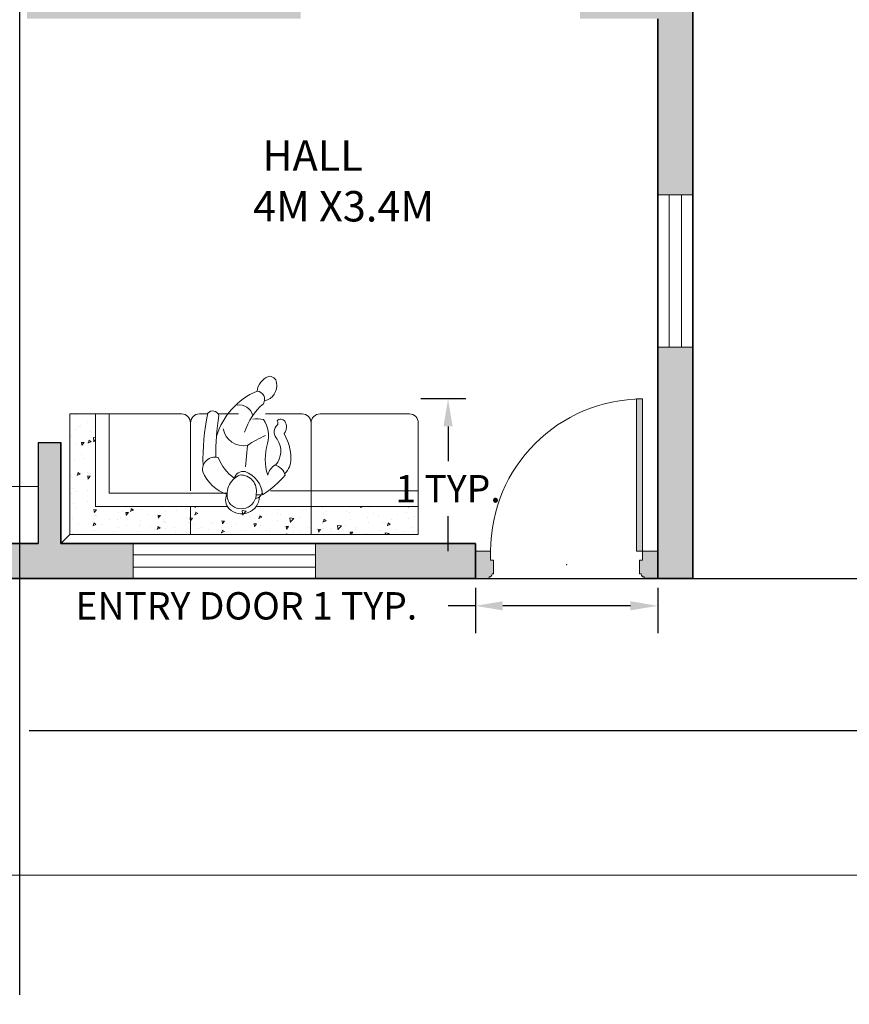
# Model space of a CAD drawing. Units: metres. Extents: x 2031 to 2061.8, y 1886.4 to 1909.8.
# Tile 5 of 10: x 2040.4 to 2045.9, y 1896.6 to 1903. Entities that reach past the tile are written whole.
import ezdxf

# ---------------------------------------------------------------- set-up
doc = ezdxf.new("R2010")
doc.units = ezdxf.units.M
for name, color, linetype, lineweight in [('A-ANNO-DIMS', 2, 'Continuous', 18), ('A-ANNO-SYMB', 7, 'Continuous', 18), ('A-AREA-IDEN', 7, 'Continuous', 18), ('A-FLOR-CASE', 8, 'Continuous', 18), ('A-WALL-PATT', 252, 'Continuous', 13), ('doors & windows', 30, 'Continuous', 18), ('furniture', 24, 'Continuous', 13), ('inner walls', 4, 'Continuous', 25), ('windows', 30, 'Continuous', 18)]:
    doc.layers.add(name, color=color, linetype=linetype, lineweight=lineweight)
doc.layers.add('outer walls', color=1, linetype='Continuous', lineweight=35, plot=False)
doc.styles.get("Standard").update_dxf_attribs({"font": 'arial.ttf'})
doc.dimstyles.get("Standard").update_dxf_attribs({"dimtxt": 0.18, "dimasz": 0.18, "dimexe": 0.18, "dimexo": 0.0625, "dimgap": 0.09, "dimtad": 0, "dimtih": 1, "dimtoh": 1, "dimdec": 4, "dimzin": 0, "dimdsep": 46, "dimtxsty": 'Standard', "dimcen": 0.09, "dimadec": 0, "dimazin": 0, "dimtfac": 1, "dimtdec": 4, "dimtofl": 0, "dimtmove": 0, "dimatfit": 3, "dimfxl": 1, "dimtolj": 1, "dimtzin": 0, "dimarcsym": 0})

# ---------------------------------------------------------------- blocks, each defined once
blk = doc.blocks.new('MAN')
at = {"layer": 'doors & windows'}
blk.add_line((1.300800906350296, -9.84959528513384), (0.8904374767287208, -5.445845033773593), dxfattribs=at)
for centre, radius, start, end in [((0.1037123764109868, 0.4753156361215943), 3.598756859045963, 2.892834703444422, 134.5528130484283), ((-0.8140254724787943, 1.304327540725086), 2.365253172473404, 132.7992866420525, 210.121851321739), ((0, 0), 3.061108984742475, 359.7942295014935, 144.0351361071093), ((-0.3633920898082081, -7.559071704207049), 8.072164320400084, 108.0152780974362, 157.572398056333), ((1.301573089887071, 0.0543302265038861), 4.161925274979446, 155.2349168989444, 248.5050710882839), ((-0.9836814564403439, 0.547290744163341), 5.343198326568241, 289.2818803665456, 356.6236969592651), ((2.859237223942386, -0.4426391913593975), 1.382894366902046, 352.7442777867131, 87.75246021842113), ((-8.985276052369024, -19.76823538750839), 24.03892498258363, 41.64703997883317, 56.30671787941347), ((-0.0988194797739439, -0.6052478084899349), 3.215301113927425, 267.7788313610161, 10.65067983897931), ((4.143205946155646, -10.81743618396086), 9.463104537162922, 125.6850708490397, 158.6986920169586), ((0.3763108145333334, -2.747678514157335), 1.794664715172271, 192.3382218214999, 283.0231027302844), ((15.87095863746732, -7.044219620172), 10.97040526684232, 162.7001941861219, 196.7262446060391), ((8.594165555367644, -3.010791798680655), 3.289009321049118, 193.5597814051185, 239.944556513456), ((5.829985165804284, -2.727362049182412), 3.323504133272041, 289.6374375416966, 341.2910971833122), ((-5.320902471805162, -4.920865143889223), 2.542708736999539, 170.0019599054575, 284.7527218828349), ((34.75273821595339, -7.193116357080249), 42.52722992385938, 177.9613012241334, 192.455084865526), ((3.83937866918498, -8.669162756695634), 4.236875526839672, 325.4362816064845, 41.84461326321779), ((6.116215034496013, -7.032657906923288), 4.013837071462978, 358.2670608736945, 46.93896446104425), ((54.7561281621764, -7.351095861722853), 59.9482441757825, 180.1043773931473, 188.2297346519416), ((-0.7768904974298892, -6.944592287015892), 10.90711801386748, 330.756224817159, 358.8996909335112), ((0.5047388683249913, -14.04557705046136), 4.270828695151803, 79.25751258177043, 168.5090206165554), ((16.49227294783997, 13.40849769215297), 27.77984362316463, 236.8486639276975, 245.4270106682865), ((9.025193711691943, -7.361610266651648), 14.71513093359242, 197.1764710295229, 246.7640806022149), ((-0.1907322920313632, -11.8133281045916), 5.784537061339297, 325.2412276434859, 16.17937157640406), ((8.85497270348916, -12.54250403754724), 2.119023409880545, 136.0875325313529, 215.1076939624027), ((12.84110766836701, -8.623294523680782), 12.77442167687985, 197.9012250797993, 229.3503854862603), ((6.795724314283273, -14.36854317724363), 0.6891912781102575, 315.9836169398009, 61.79474043932597), ((7.062938957867345, -13.61414320857268), 2.147447575500176, 328.4118945862401, 38.64735298079067), ((-5.78012869004862, -15.61065174797719), 1.247517943767832, 217.2140234901752, 345.0613840222), ((-0.400707327332418, -15.26883761241566), 2.808757651487922, 261.6004897306414, 345.5997888512171), ((3.211235571911339, -8.720384485263041), 6.531946877074549, 262.8142164373346, 281.9310149491412), ((8.045979600851894, -14.11708026683455), 1.050184368679085, 224.0635746420259, 323.6869684137312), ((3.089333312178894, -19.20433111995709), 1.68390170903289, 274.4439678377158, 31.86589660260227), ((4.090151064548964, -22.00922691863412), 3.160356054196907, 349.1500221718577, 77.97162169367246), ((6.986801406002953, -20.3553233934708), 3.803794739384279, 187.9765915169998, 248.0432243045189), ((5.750086688982904, -22.44212759914928), 1.452983263573688, 262.6631028846992, 353.5985654676438)]:
    blk.add_arc(centre, radius, start, end, dxfattribs=at)
blk = doc.blocks.new('sofa 2')
at = {"layer": 'furniture', "ltscale": 0.5}
h = blk.add_hatch(dxfattribs=at)
h.set_pattern_fill('AR-CONC', color=256, angle=450, style=0)
h.set_pattern_definition([(40, (-1099.150670582166, 871.6550217453555), (-0.6275213498259516, 7.172601826007534), [0.7499999999999992, -8.249999999999988]), (94.99999999999999, (-1099.150670582166, 871.6550217453555), (7.521921337000118, -1.387513336129999), [0.6, -6.599999999999999]), (349.5486, (-1099.202963982166, 872.2527385453554), (6.894395420609535, 5.785093817140215), [0.6374019000000001, -7.011421119999999]), (43.81579999999999, (-1097.150670582165, 871.6550217453555), (-1.655190143290181, 10.67241048625644), [1.124999999999999, -12.375]), (353.3644, (-1097.288603652166, 872.5443891953554), (9.741178709004418, 9.346627055487033), [0.9561028799999983, -10.51712999999997]), (98.81580000000002, (-1097.150670582165, 871.6550217453555), (9.741186009253246, 9.34661945133627), [0.9, -9.899999999999999]), (69.00000000000001, (-1097.650670582166, 872.6550217453555), (-4.026188906653388, 5.969070521184616), [0.75, -8.249999999999998]), (124, (-1097.650670582166, 872.6550217453555), (7.25150045046853, 2.433153319215817), [0.5999999999999999, -6.599999999999998]), (18.54859999999996, (-1097.986186642165, 873.1524440753556), (3.225304967099523, 8.4022262858149), [0.6374018999999995, -7.011421119999994]), (52.49999999999997, (-1099.150670582166, 871.6550217453555), (3.328938538313114, 0.1215985531729069), [0, -6.519999999999997, 0, -6.699999999999998, 0, -6.624999999999998]), (82.5, (-1099.150670582166, 871.6550217453555), (3.944117118823602, 2.630695374421486), [0, -3.819999999999999, 0, -6.369999999999999, 0, -2.524999999999999]), (122.5, (-1099.150670582166, 869.4250217453555), (-0.2255487173437983, 5.33822436172409), [0, -2.5, 0, -7.799999999999999, 0, -10.35]), (132.5, (-1099.150670582166, 868.4250217453554), (1.001049823323175, 5.831861693423862), [0, -3.25, 0, -5.179999999999999, 0, -7.349999999999999])])
h.paths.add_polyline_path([(-8.269725417867454, -37.69644211528794, 0.1688724756547801), (-7.901216225471903, -36.75698787828117, 0.6138083482869159), (-6.947255836040998, -30.76691878839267, 0.0748688598940706), (-8.26972541786768, -30.38266280423341), (-8.26972541786768, -28.99999999999989), (-1.999999999999776, -29), (-1.999999999999779, -56.00000000000012), (-8.269725417867456, -56)])
h.paths.add_polyline_path([(-8.26972541786745, -7.765106587653121), (-29, -7.765106587653118), (-29, -1.999999999999996), (-2, -1.999999999999999), (-1.999999999999776, -28.99999999999989), (-8.26972541786768, -29)])
h.paths.add_polyline_path([(-8.269725417867459, -80.00000000000023), (-1.999999999999782, -80.00000000000033), (-1.999999999999779, -56.00000000000012), (-8.269725417867456, -56.00000000000012)])
at = {"layer": 'furniture'}
for p, q in [((-2, -1.999999999999999), (0, 0)), ((-29, -2.000000000000053), (-2, -1.999999999999999)), ((-29.00000000000023, -26.99999999999954), (-29, -1.999999999999882)), ((-2, -1.999999999999999), (-1.999999999999782, -80.00000000000033)), ((-8.269725417867678, -7.765106587653121), (-29.00000000000011, -7.765106587653118)), ((-8.269725417867681, -37.2693090459178), (-8.269725417867678, -7.765106587653121)), ((-11.26972541786768, -10.76510658765312), (-29.00000000000011, -10.76510658765312)), ((-11.26972541786768, -37.2693090459178), (-11.26972541786768, -10.76510658765312)), ((-27.00000000000046, -28.99999999999954), (-11.7952580518181, -29.00000000000011)), ((-8.26972541786768, -29), (-2.000000000000003, -29)), ((-29.00000000000011, -32.86544848654179), (-29, -30.99999999999943)), ((-29.0000000000005, -39.73699459320184), (-29.00000000000024, -35.16470018482259)), ((-8.269725417867454, -37.69644211528794), (-8.269725417867454, -37.69801474660262)), ((-8.269725417867454, -43.65667845911833), (-8.269725417867459, -80.00000000000023)), ((-29.00000000000001, -45.79600710233531), (-29.00000000000001, -53.99999999999988)), ((-11.79525805181789, -80.00000000000033), (-11.79525805181809, -46.88939649664059)), ((-27.00000000000001, -55.99999999999977), (-2.000000000000234, -56.00000000000012)), ((-29.00000000000001, -77.99999999999989), (-29.00000000000001, -57.99999999999977)), ((-1.999999999999782, -80.00000000000033), (-27.00000000000001, -79.99999999999989))]:
    blk.add_line(p, q, dxfattribs=at)
for centre, start, end in [((-27.00000000000023, -26.99999999999954), 180, 270), ((-27.00000000000001, -30.99999999999954), 89.99999999999999, 180), ((-27.00000000000001, -53.99999999999988), 180, 270), ((-27.00000000000001, -57.99999999999977), 89.99999999999999, 180), ((-27.00000000000001, -77.99999999999989), 180, 270)]:
    blk.add_arc(centre, 2, start, end, dxfattribs=at)
at = {"xscale": 1.099999999999999, "yscale": 1.099999999999999, "zscale": 1.099999999999999, "rotation": 270}
blk.add_blockref('MAN', (-11.1253145417007, -40.34430049627808), dxfattribs=at)
blk = doc.blocks.new('D2')
at = {"layer": 'doors & windows'}
h = blk.add_hatch(dxfattribs=at)
h.set_pattern_fill('DOTS', color=256, scale=2, angle=180, style=0)
h.set_pattern_definition([(180, (0, -3.999999999998181), (-0.0625, -0.125), [0, -0.125])])
h.paths.add_polyline_path([(2.5, 1.819e-12), (3.5, 1.819e-12), (3.500000000001818, 24.97999199359535, 0.0100030022021123), (2.500000000001818, 25.00000000000182)])
h = blk.add_hatch(dxfattribs=at)
h.set_pattern_fill('DOTS', color=256, scale=2, angle=180, style=0)
h.set_pattern_definition([(180, (0, 0), (-0.0625, -0.125), [0, -0.125])])
edge = h.paths.add_edge_path()
edge.add_line((27.50000000000182, 1.819e-12), (27.50000000000182, -1.499999999998181))
edge.add_line((27.50000000000182, -1.499999999998181), (27.00000000000157, -1.499999999998181))
edge.add_line((27.00000000000157, -1.499999999998181), (27.00000000000039, -3.749999999998181))
edge.add_line((27.00000000000039, -3.749999999998181), (27.25, -3.749999999998181))
edge.add_arc((27.75893604593965, -3.741063954058532), 0.5090144907305875, 181.0059124648427, 268.9940875351573)
edge.add_line((27.75, -4.249999999998181), (27.75, -4.499999999998181))
edge.add_line((27.75, -4.499999999998181), (30.00000000000182, -4.499999999998181))
edge.add_line((30.00000000000182, -4.499999999998181), (30.00000000000182, 0))
edge.add_line((30.00000000000182, 0), (27.50000000000182, 1.819e-12))
edge = h.paths.add_edge_path()
edge.add_line((2.5, -1.499999999998181), (2.5, 1.819e-12))
edge.add_line((2.5, 1.819e-12), (1.819e-12, 0))
edge.add_line((1.819e-12, 0), (0, -4.499999999998181))
edge.add_line((0, -4.499999999998181), (2.250000000001548, -4.499999999998181))
edge.add_line((2.250000000001548, -4.499999999998181), (2.250000000001548, -4.249999999998181))
edge.add_arc((2.2410639540619, -3.741063954058532), 0.5090144907305875, 271.0059124648427, 358.9940875351573)
edge.add_line((2.750000000001548, -3.749999999998181), (3, -3.749999999998181))
edge.add_line((3, -3.749999999998181), (3, -1.499999999998181))
edge.add_line((3, -1.499999999998181), (2.5, -1.499999999998181))
for p, q in [((1.819e-12, 0), (0, -4.499999999998181)), ((30.00000000000182, 0), (30.00000000000182, -4.499999999998181))]:
    blk.add_line(p, q)
blk.add_lwpolyline([(3.5, 1.819e-12), (3.500000000001818, 25.00000000000182), (2.500000000001818, 25.00000000000182), (2.5, 1.819e-12)], close=True, dxfattribs=at)
for points in [[(3, -3.749999999998181), (3, -1.499999999998181), (2.5, -1.499999999998181), (2.5, 1.819e-12), (1.819e-12, 0)], [(27.00000000000039, -3.749999999998181), (27.00000000000182, -1.499999999998181), (27.50000000000182, -1.499999999998181), (27.50000000000182, 1.819e-12), (30, 0)], [(0, -4.499999999998181), (2.250000000001548, -4.499999999998181)], [(30, -4.499999999998181), (27.75, -4.499999999998181)]]:
    blk.add_lwpolyline(points, dxfattribs=at)
for points in [[(2.250000000001548, -4.499999999998181), (2.250000000001548, -4.249999999998181, 0.4039662087126686), (2.750000000001548, -3.749999999998181), (3.000000000001548, -3.749999999998181)], [(27.75, -4.499999999998181), (27.75, -4.249999999998181, -0.4039662087126686), (27.25, -3.749999999998181), (27, -3.749999999998181)]]:
    blk.add_lwpolyline(points, format="xyb", dxfattribs=at)
at = {"layer": 'doors & windows', "ltscale": 6}
blk.add_arc((2.5, 1.819e-12), 25, 0, 90, dxfattribs=at)
at = {"layer": 'doors & windows'}
blk.add_point((15, -2.24999999999909), dxfattribs=at)
blk = doc.blocks.new('WIN-1200')
for p, q in [((0.2299999999995634, 1.200000000000045), (-4.547e-13, 1.199999999999818)), ((0.0750000000007276, -2.274e-13), (0.0749999999995907, 1.200000000000045)), ((0.1550000000006548, -2.274e-13), (0.154999999999518, 1.200000000000045)), ((0.2300000000007003, 0), (6.821e-13, -2.274e-13))]:
    blk.add_line(p, q)
blk = doc.blocks.new('WIN-1000')
for p, q in [((2.274e-13, 0), (0, 0.2299999999997908)), ((1.000000000000227, 9.095e-13), (1, 0.2300000000007003)), ((2.274e-13, 0.1549999999997453), (1.000000000000227, 0.1549999999997453)), ((2.274e-13, 0.0749999999998181), (1.000000000000227, 0.0749999999998181))]:
    blk.add_line(p, q)
blk = doc.blocks.new('*D18')
at = {"layer": 'A-ANNO-DIMS', "color": 0, "lineweight": -2, "transparency": 16777216}
for p, q in [((2043.413579428145, 1899.308702985826), (2043.413579428145, 1899.011202985826)), ((2044.613579428145, 1899.308702985826), (2044.613579428145, 1899.011202985826)), ((2043.413579428145, 1899.191202985826), (2043.233579428145, 1899.191202985826)), ((2044.433579428145, 1899.191202985826), (2043.593579428145, 1899.191202985826))]:
    blk.add_line(p, q, dxfattribs=at)
at = {"layer": 'A-ANNO-DIMS', "color": 0, "transparency": 16777216}
for points in [[(2043.593579428145, 1899.221202985826), (2043.593579428145, 1899.161202985826), (2043.413579428145, 1899.191202985826)], [(2044.433579428145, 1899.221202985826), (2044.433579428145, 1899.161202985826), (2044.613579428145, 1899.191202985826)]]:
    blk.add_solid(points, dxfattribs=at)
at = {"layer": 'Defpoints', "color": 0, "transparency": 16777216}
for p in [(2043.413579428145, 1899.371202985826), (2044.613579428145, 1899.371202985826), (2043.413579428145, 1899.191202985826)]:
    blk.add_point(p, dxfattribs=at)
at = {"layer": 'A-ANNO-DIMS', "color": 0, "transparency": 16777216, "insert": (2041.906969605499, 1899.191202985826), "char_height": 0.18, "attachment_point": 5}
blk.add_mtext('\\A1;ENTRY DOOR 1 TYP.', dxfattribs=at)
blk = doc.blocks.new('*D19')
at = {"layer": 'A-ANNO-DIMS', "color": 0, "lineweight": -2, "transparency": 16777216}
for p, q in [((2043.351079428146, 1900.551202985827), (2043.053579428146, 1900.551202985827)), ((2043.233579428147, 1900.371202985827), (2043.233579428147, 1900.141632726618)), ((2043.233579428147, 1899.551202985827), (2043.233579428147, 1899.780773245035)), ((2043.351079428146, 1899.371202985827), (2043.053579428146, 1899.371202985827))]:
    blk.add_line(p, q, dxfattribs=at)
at = {"layer": 'A-ANNO-DIMS', "color": 0, "transparency": 16777216}
for points in [[(2043.203579428147, 1900.371202985827), (2043.263579428147, 1900.371202985827), (2043.233579428147, 1900.551202985827)], [(2043.203579428147, 1899.551202985827), (2043.263579428147, 1899.551202985827), (2043.233579428147, 1899.371202985827)]]:
    blk.add_solid(points, dxfattribs=at)
at = {"layer": 'Defpoints', "color": 0, "transparency": 16777216}
for p in [(2043.233579428147, 1900.551202985827), (2043.413579428146, 1900.551202985827), (2043.413579428146, 1899.371202985827)]:
    blk.add_point(p, dxfattribs=at)
at = {"layer": 'A-ANNO-DIMS', "color": 0, "transparency": 16777216, "insert": (2043.233579428147, 1899.961202985825), "char_height": 0.18, "attachment_point": 5}
blk.add_mtext('\\A1;1 TYP.', dxfattribs=at)
blk = doc.blocks.new('*D44')
at = {"layer": 'A-ANNO-DIMS', "color": 0, "lineweight": -2, "transparency": 16777216}
for p, q in [((2036.232783, 1900.719895), (2036.232783, 1886.390195)), ((2056.453886, 1889.9931), (2056.453886, 1886.390195)), ((2036.412783, 1886.570195), (2045.94901662824, 1886.570195)), ((2056.273886, 1886.570195), (2046.73765237176, 1886.570195))]:
    blk.add_line(p, q, dxfattribs=at)
at = {"layer": 'A-ANNO-DIMS', "color": 0, "transparency": 16777216}
for points in [[(2036.412783, 1886.600195), (2036.412783, 1886.540195), (2036.232783, 1886.570195)], [(2056.273886, 1886.600195), (2056.273886, 1886.540195), (2056.453886, 1886.570195)]]:
    blk.add_solid(points, dxfattribs=at)
at = {"layer": 'Defpoints', "color": 0, "transparency": 16777216}
for p in [(2036.232783, 1900.782395), (2056.453886, 1890.0556), (2056.453886, 1886.570195)]:
    blk.add_point(p, dxfattribs=at)
at = {"layer": 'A-ANNO-DIMS', "color": 0, "transparency": 16777216, "insert": (2046.3433345, 1886.570195), "char_height": 0.18, "attachment_point": 5}
blk.add_mtext('\\A1;20.22', dxfattribs=at)
blk = doc.blocks.new('*D57')
at = {"layer": 'A-ANNO-DIMS', "color": 0, "lineweight": -2, "transparency": 16777216}
for p, q in [((2040.478205000001, 1899.371213000001), (2061.614374000002, 1899.371213000001)), ((2061.434374000002, 1899.191213), (2061.434374000002, 1899.05158134925)), ((2061.434374000002, 1898.551213000001), (2061.434374000002, 1898.690844650751)), ((2040.478205000001, 1898.371213), (2061.614374000002, 1898.371213))]:
    blk.add_line(p, q, dxfattribs=at)
at = {"layer": 'A-ANNO-DIMS', "color": 0, "transparency": 16777216}
for points in [[(2061.404374000002, 1899.191213), (2061.464374000002, 1899.191213), (2061.434374000002, 1899.371213000001)], [(2061.404374000002, 1898.551213000001), (2061.464374000002, 1898.551213000001), (2061.434374000002, 1898.371213)]]:
    blk.add_solid(points, dxfattribs=at)
at = {"layer": 'Defpoints', "color": 0, "transparency": 16777216}
for p in [(2040.415705000001, 1899.371213000001), (2061.434374000002, 1899.371213000001), (2040.415705000001, 1898.371213)]:
    blk.add_point(p, dxfattribs=at)
at = {"layer": 'A-ANNO-DIMS', "color": 0, "transparency": 16777216, "insert": (2061.434374000002, 1898.871212999999), "char_height": 0.18, "attachment_point": 5}
blk.add_mtext('\\A1;1', dxfattribs=at)
blk = doc.blocks.new('*D58')
at = {"layer": 'A-ANNO-DIMS', "color": 0, "lineweight": -2, "transparency": 16777216}
for p, q in [((2040.415705, 1896.633713), (2040.415705, 1909.84065)), ((2052.040038, 1896.633713), (2052.040038, 1909.84065)), ((2040.595705, 1909.66065), (2045.773082959755, 1909.66065)), ((2051.860038, 1909.66065), (2046.682660040246, 1909.66065))]:
    blk.add_line(p, q, dxfattribs=at)
at = {"layer": 'A-ANNO-DIMS', "color": 0, "transparency": 16777216}
for points in [[(2040.595705, 1909.69065), (2040.595705, 1909.63065), (2040.415705, 1909.66065)], [(2051.860038, 1909.69065), (2051.860038, 1909.63065), (2052.040038, 1909.66065)]]:
    blk.add_solid(points, dxfattribs=at)
at = {"layer": 'Defpoints', "color": 0, "transparency": 16777216}
for p in [(2052.040038, 1909.66065), (2040.415705, 1896.571213), (2052.040038, 1896.571213)]:
    blk.add_point(p, dxfattribs=at)
at = {"layer": 'A-ANNO-DIMS', "color": 0, "transparency": 16777216, "insert": (2046.227871500001, 1909.66065), "char_height": 0.18, "attachment_point": 5}
blk.add_mtext('\\A1;11.624', dxfattribs=at)

msp = doc.modelspace()

# ---------------------------------------------------------------- hatches: boundary and pattern name
at = {"layer": 'A-WALL-PATT'}
h = msp.add_hatch(color=256, dxfattribs=at)
h.dxf.hatch_style = 1
h.paths.add_polyline_path([(2044.843886051581, 1905.431202972395), (2043.662726773602, 1905.431202972395), (2043.662726773602, 1905.201202972395), (2044.613886051581, 1905.201202972395), (2044.613886051581, 1903.201202972395), (2044.10203621828, 1903.201202972395), (2044.10203621828, 1903.051247813867), (2044.613886051581, 1903.051202972395), (2044.613784550147, 1901.892599367488), (2044.843481671829, 1901.892599367488)])
h.paths.add_polyline_path([(2044.843886051581, 1907.081202972395), (2044.693886051581, 1907.081202972395), (2044.693886051581, 1905.431202972395), (2044.843886051581, 1905.431202972395)])
h.paths.add_polyline_path([(2042.662726773602, 1905.431202972395), (2041.608725591668, 1905.431202972395), (2041.608725591668, 1905.201202972395), (2042.113886051581, 1905.201202972395), (2042.113886051581, 1903.201202972395), (2042.11388605158, 1903.200960518025), (2041.878665859902, 1903.200960518025, -0.0160568248018428), (2041.87111792116, 1903.201202972395), (2040.613886051581, 1903.201202972395), (2040.463886051581, 1903.201202972395), (2040.46388605158, 1903.051202972395), (2042.263886051581, 1903.051202972395), (2042.263886051581, 1905.201202972395), (2042.662726773602, 1905.201202972395)])
h.paths.add_polyline_path([(2040.804457664849, 1903.878793012381), (2041.776183449296, 1903.878793012381), (2041.776183449296, 1904.438513339803), (2040.804457664849, 1904.438513339803)], flags=25)
h.paths.add_polyline_path([(2042.05521314868, 1900.945611707966), (2043.754121743495, 1900.945611707966), (2043.754121743495, 1901.691905477861), (2042.05521314868, 1901.691905477861)], flags=9)
h.paths.add_polyline_path([(2038.540886554753, 1905.248744193212), (2040.159440442883, 1905.248744193212), (2040.159440442883, 1905.995037963107), (2038.540886554753, 1905.995037963107)], flags=9)
h.paths.add_polyline_path([(2038.693906317999, 1902.140700941841), (2040.392814912815, 1902.140700941841), (2040.392814912815, 1902.886994711737), (2038.693906317999, 1902.886994711737)], flags=9)
h.paths.add_polyline_path([(2042.359230799286, 1903.821641126969), (2043.685560949354, 1903.821641126969), (2043.685560949354, 1904.567934896864), (2042.359230799286, 1904.567934896864)], flags=9)
h = msp.add_hatch(color=256, dxfattribs=at)
h.dxf.hatch_style = 1
h.paths.add_polyline_path([(2044.843367395183, 1900.892599367488), (2044.61369694345, 1900.892599367488), (2044.61356365894, 1899.371202985826), (2044.843193535108, 1899.371202985826)])
h.paths.add_polyline_path([(2041.161147521447, 1899.371202985826), (2041.161147521447, 1899.601202985826), (2040.68737920617, 1899.601202985827), (2040.68737920617, 1899.976202985826), (2040.687485090836, 1900.265858024963), (2040.53737920617, 1900.265912896825), (2040.53737920617, 1899.601202985826), (2038.113193535108, 1899.601202985827), (2038.112783035539, 1900.932395301215), (2036.462783035539, 1900.932395301215), (2036.463068993382, 1901.839002867159), (2036.233083640793, 1901.839002867159), (2036.232783035539, 1900.782395301215), (2037.962783035539, 1900.782395301215), (2037.963193535108, 1899.371202985826)])
h = msp.add_hatch(color=256, dxfattribs=at)
h.dxf.hatch_style = 1
h.paths.add_polyline_path([(2043.413579428145, 1899.371202985826), (2043.413579428145, 1899.551202985826), (2043.414968643082, 1899.601202985826), (2042.361147521447, 1899.601202985826), (2042.361147521447, 1899.371202985826)])
edge = h.paths.add_edge_path()
edge.add_line((2038.506381150364, 1899.788201292628), (2039.966159003426, 1899.788201292628))
edge = h.paths.add_edge_path()
edge.add_line((2039.966159003426, 1899.766083446369), (2038.506381150364, 1899.766083446369))
edge = h.paths.add_edge_path()
edge.add_arc((2038.528498996622, 1899.630681587596), 0.0294356005293348, 221.2883925659197, 318.7116074340803)
edge = h.paths.add_edge_path()
edge.add_arc((2038.572734689139, 1899.933839879253), 0.0239496954881524, 22.5548696809955, 157.4451303190045)
edge = h.paths.add_edge_path()
edge.add_line((2038.506381150364, 1899.61125852256), (2038.594852535398, 1899.943026216438))
edge = h.paths.add_edge_path(flags=17)
edge.add_line((2038.550616842881, 1899.61125852256), (2038.550616842881, 1899.943026216438))
edge = h.paths.add_edge_path()
edge.add_arc((2038.639088227915, 1899.630681587596), 0.0294356005293348, 221.2883925659197, 318.7116074340803)
edge = h.paths.add_edge_path()
edge.add_arc((2038.683323920432, 1899.933839879253), 0.0239496954881524, 22.5548696809955, 157.4451303190045)
edge = h.paths.add_edge_path()
edge.add_line((2038.616970381656, 1899.61125852256), (2038.70544176669, 1899.943026216438))
edge = h.paths.add_edge_path(flags=17)
edge.add_line((2038.661206074174, 1899.61125852256), (2038.661206074174, 1899.943026216438))
edge = h.paths.add_edge_path()
edge.add_arc((2038.749677459207, 1899.630681587596), 0.0294356005293348, 221.2883925659197, 318.7116074340803)
edge = h.paths.add_edge_path()
edge.add_arc((2038.793913151724, 1899.933839879253), 0.0239496954881524, 22.5548696809955, 157.4451303190045)
edge = h.paths.add_edge_path()
edge.add_line((2038.727559612949, 1899.61125852256), (2038.816030997983, 1899.943026216438))
edge = h.paths.add_edge_path(flags=17)
edge.add_line((2038.771795305466, 1899.61125852256), (2038.771795305466, 1899.943026216438))
edge = h.paths.add_edge_path()
edge.add_arc((2039.678627002065, 1899.630681587596), 0.0294356005293348, 221.2883925659197, 318.7116074340803)
edge = h.paths.add_edge_path()
edge.add_arc((2039.722862694583, 1899.933839879253), 0.0239496954881524, 22.5548696809955, 157.4451303190045)
edge = h.paths.add_edge_path()
edge.add_line((2039.656509155807, 1899.61125852256), (2039.744980540841, 1899.943026216438))
edge = h.paths.add_edge_path(flags=17)
edge.add_line((2039.700744848324, 1899.61125852256), (2039.700744848324, 1899.943026216438))
edge = h.paths.add_edge_path()
edge.add_arc((2039.789216233358, 1899.630681587596), 0.0294356005293348, 221.2883925659197, 318.7116074340803)
edge = h.paths.add_edge_path()
edge.add_arc((2039.833451925875, 1899.933839879253), 0.0239496954881524, 22.5548696809955, 157.4451303190045)
edge = h.paths.add_edge_path()
edge.add_line((2039.7670983871, 1899.61125852256), (2039.855569772134, 1899.943026216438))
edge = h.paths.add_edge_path(flags=17)
edge.add_line((2039.811334079616, 1899.61125852256), (2039.811334079616, 1899.943026216438))
edge = h.paths.add_edge_path()
edge.add_arc((2039.899805464651, 1899.630681587596), 0.0294356005293348, 221.2883925659197, 318.7116074340803)
edge = h.paths.add_edge_path()
edge.add_arc((2039.944041157168, 1899.933839879253), 0.0239496954881524, 22.5548696809955, 157.4451303190045)
edge = h.paths.add_edge_path()
edge.add_line((2039.877687618392, 1899.61125852256), (2039.966159003426, 1899.943026216438))
edge = h.paths.add_edge_path(flags=17)
edge.add_line((2039.921923310909, 1899.61125852256), (2039.921923310909, 1899.943026216438))
h.paths.add_polyline_path([(2038.837326301555, 1899.786483056072), (2039.659277368514, 1899.786483056072), (2039.659277368514, 1899.923716295886), (2038.837326301555, 1899.923716295886)], flags=9)

# ---------------------------------------------------------------- linework, layer by layer
at = {"layer": 'A-ANNO-SYMB'}
msp.add_line((2033.125780009863, 1897.420015762724), (2060.053374346622, 1897.420015762724), dxfattribs=at)
at = {"layer": 'A-FLOR-CASE', "ltscale": 0.3}
msp.add_line((2038.113193535108, 1899.976202985826), (2040.53737920617, 1899.976202985826), dxfattribs=at)
at = {"layer": 'furniture'}
msp.add_line((2041.971391056426, 1899.92), (2042.003877577646, 1899.92), dxfattribs=at)
at = {"layer": 'inner walls'}
for q in [(2040.53737920617, 1899.601202985826), (2040.68737920617, 1900.26585806367)]:
    msp.add_line((2040.53737920617, 1900.265912896825), q, dxfattribs=at)
at = {"layer": 'outer walls'}
for p, q in [((2044.843886051581, 1905.431202972395), (2044.843193535108, 1899.371202985826)), ((2044.613886051581, 1903.051202972395), (2044.61356365894, 1899.371202985826)), ((2038.113193535108, 1899.601202985827), (2040.537242123281, 1899.601202985826)), ((2043.414968643082, 1899.371202985826), (2043.414968643082, 1899.601202985826)), ((2037.963193535108, 1899.371202985826), (2043.414968643082, 1899.371202985826)), ((2044.524968643081, 1899.371202985826), (2044.843193535108, 1899.371202985826))]:
    msp.add_line(p, q, dxfattribs=at)
msp.add_lwpolyline([(2043.414968643082, 1899.601202985826), (2040.68737920617, 1899.601202985827), (2040.68737920617, 1899.976202985826), (2040.687485090836, 1900.265858024963)], dxfattribs=at)

# ---------------------------------------------------------------- block references
at = {"layer": 'doors & windows', "xscale": -0.0399999999999984, "yscale": 0.0399999999999984, "zscale": 0.0399999999999984}
msp.add_blockref('D2', (2044.613579428145, 1899.551202985826), dxfattribs=at)
at = {"layer": 'furniture', "xscale": -0.0293822575608255, "yscale": 0.0293822575608255, "zscale": 0.0293822575608255, "rotation": 90}
msp.add_blockref('sofa 2', (2040.687379206171, 1899.601202985826), dxfattribs=at)
at = {"layer": 'windows'}
for name, p, rotation in [('WIN-1000', (2044.613367395184, 1901.892599367488), 269.9999999999067), ('WIN-1200', (2042.361147521447, 1899.371202985824), 89.99999999997905)]:
    msp.add_blockref(name, p, dxfattribs=dict(at, rotation=rotation))

# ---------------------------------------------------------------- texts
at = {"layer": 'A-AREA-IDEN', "insert": (2041.767631281673, 1901.718280378523), "char_height": 0.2, "attachment_point": 7}
msp.add_mtext_dynamic_manual_height_columns('    HALL\\P   4M X3.4M', width=2.302330104705106, gutter_width=12.5, heights=[0], dxfattribs=at)

# ---------------------------------------------------------------- dimensions: what is measured, and where the dimension line sits
at = {"layer": 'A-ANNO-DIMS'}
for base, p1, p2, override, picture, middle in [((2052.040038, 1909.66065), (2040.415705, 1896.571213), (2052.040038, 1896.571213), {"dimdec": 3, "dimlfac": 1, "dimrnd": 0, "dimzin": 0, "dimdsep": 46, "dimlunit": 2}, '*D58', (2046.227871500001, 1909.66065)), ((2056.453886, 1886.570195), (2036.232783, 1900.782395), (2056.453886, 1890.0556), {"dimdec": 2, "dimlfac": 1, "dimrnd": 0, "dimzin": 0, "dimdsep": 46, "dimlunit": 2}, '*D44', (2046.3433345, 1886.570195))]:
    dim = msp.add_linear_dim(base=base, p1=p1, p2=p2, dimstyle='Standard', override=override, dxfattribs=at)
    dim.commit()
    dim.dimension.update_dxf_attribs({"geometry": picture, "text_midpoint": middle})
for base, p1, p2, angle, text, picture, middle in [((2043.233579428147, 1900.551202985827), (2043.413579428145, 1899.371202985826), (2043.413579428145, 1900.551202985826), 90, '<> TYP.', '*D19', (2043.233579428147, 1899.961202985825)), ((2043.413579428145, 1899.191202985826), (2044.613579428145, 1899.371202985826), (2043.413579428145, 1899.371202985826), 180, 'ENTRY DOOR <> TYP.', '*D18', (2041.906969605499, 1899.191202985826))]:
    dim = msp.add_linear_dim(base=base, p1=p1, p2=p2, angle=angle, text=text, dimstyle='Standard', override={"dimdec": 0, "dimlfac": 1, "dimrnd": 0, "dimzin": 0, "dimdsep": 46, "dimlunit": 2}, dxfattribs=at)
    dim.commit()
    dim.dimension.update_dxf_attribs({"geometry": picture, "text_midpoint": middle})
dim = msp.add_linear_dim(base=(2061.434374000002, 1899.371213000001), p1=(2040.415705, 1898.371213), p2=(2040.415705, 1899.371213), angle=90, dimstyle='Standard', override={"dimdec": 0, "dimlfac": 1, "dimrnd": 0, "dimzin": 0, "dimdsep": 46, "dimlunit": 2}, dxfattribs=at)
dim.commit()
dim.dimension.update_dxf_attribs({"geometry": '*D57', "text_midpoint": (2061.434374000002, 1898.871212999999)})

doc.saveas('drawing.dxf')
